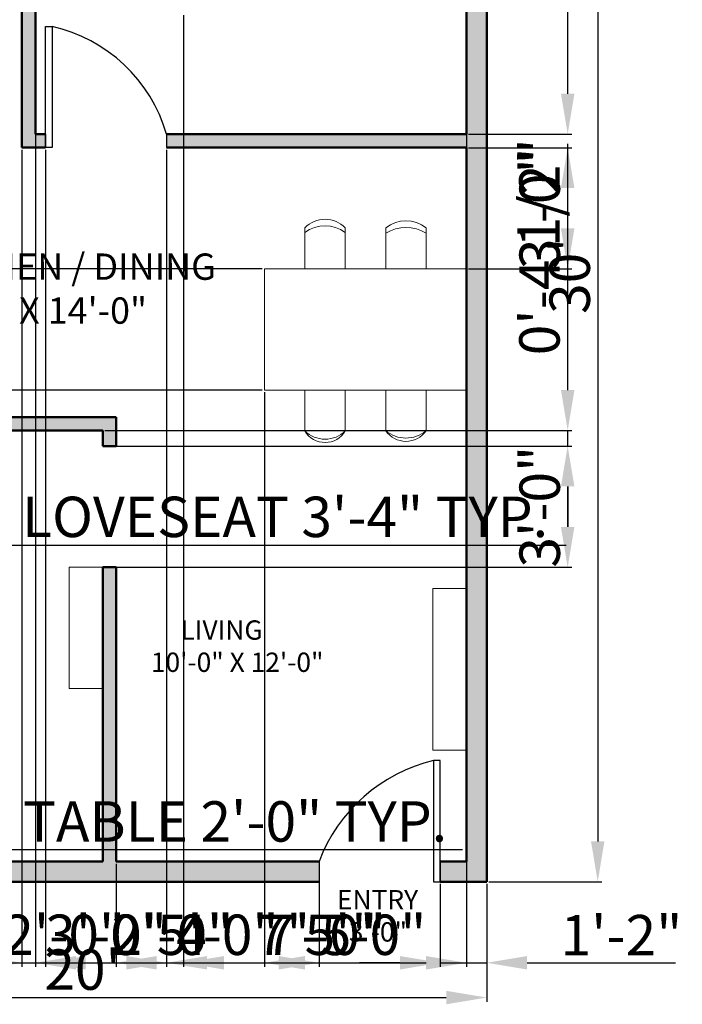
# Model space of a CAD drawing. Units: inches. Extents: x 2549 to 2991, y 1646 to 2183.
# Tile 2 of 3: x 2727 to 2924, y 1646 to 1938. Entities that reach past the tile are written whole.
import ezdxf

# ---------------------------------------------------------------- set-up
doc = ezdxf.new("R2010")
doc.units = ezdxf.units.IN
for name, color, linetype, lineweight in [('A-ANNO-DIMS', 2, 'Continuous', 18), ('A-ANNO-TEXT', 7, 'Continuous', 18), ('A-AREA-IDEN', 7, 'Continuous', 25), ('A-DOOR', 3, 'Continuous', 25), ('A-FURN', 9, 'Continuous', 18), ('A-WALL', 7, 'Continuous', 50)]:
    doc.layers.add(name, color=color, linetype=linetype, lineweight=lineweight)
doc.layers.add('A-WALL-PATT', color=251, linetype='Continuous', lineweight=13, true_color=0x636466)
doc.styles.get("Standard").update_dxf_attribs({"font": 'arial.ttf'})
doc.dimstyles.new('ISO-25', dxfattribs={"dimtxt": 12, "dimasz": 12, "dimexe": 1.25, "dimexo": 0.625, "dimtad": 1, "dimlunit": 3, "dimtxsty": 'Standard', "dimcen": 2.5, "dimadec": 0, "dimazin": 0, "dimtfac": 1, "dimtmove": 0, "dimatfit": 3, "dimfxl": 1, "dimarcsym": 0})

# ---------------------------------------------------------------- blocks, each defined once
blk = doc.blocks.new('*D5')
at = {"layer": 'A-ANNO-DIMS', "color": 0, "lineweight": -2, "transparency": 16777216}
for p, q in [((2866.66, 2042.26), (2900.26, 2042.26)), ((2899.01, 2030.26), (2899.01, 1694.26)), ((2866.66, 1682.26), (2900.26, 1682.26))]:
    blk.add_line(p, q, dxfattribs=at)
at = {"layer": 'A-ANNO-DIMS', "color": 0, "transparency": 16777216}
for points in [[(2897.01, 2030.26), (2901.01, 2030.26), (2899.01, 2042.26)], [(2897.01, 1694.26), (2901.01, 1694.26), (2899.01, 1682.26)]]:
    blk.add_solid(points, dxfattribs=at)
at = {"layer": 'Defpoints', "color": 0, "transparency": 16777216}
for p in [(2866.04, 2042.26), (2866.04, 1682.26), (2899.01, 1682.26)]:
    blk.add_point(p, dxfattribs=at)
at = {"layer": 'A-ANNO-DIMS', "color": 0, "transparency": 16777216, "insert": (2892.25, 1862.26), "char_height": 12, "attachment_point": 5, "rotation": 90}
blk.add_mtext("30'", dxfattribs=at)
blk = doc.blocks.new('*D13')
at = {"layer": 'A-ANNO-DIMS', "color": 0, "lineweight": -2, "transparency": 16777216}
for p, q in [((2626.04, 1681.64), (2626.04, 1646.63)), ((2866.04, 1681.64), (2866.04, 1646.63)), ((2638.04, 1647.88), (2854.04, 1647.88))]:
    blk.add_line(p, q, dxfattribs=at)
at = {"layer": 'A-ANNO-DIMS', "color": 0, "transparency": 16777216}
for points in [[(2638.04, 1649.88), (2638.04, 1645.88), (2626.04, 1647.88)], [(2854.04, 1649.88), (2854.04, 1645.88), (2866.04, 1647.88)]]:
    blk.add_solid(points, dxfattribs=at)
at = {"layer": 'Defpoints', "color": 0, "transparency": 16777216}
for p in [(2626.04, 1682.26), (2866.04, 1682.26), (2866.04, 1647.88)]:
    blk.add_point(p, dxfattribs=at)
at = {"layer": 'A-ANNO-DIMS', "color": 0, "transparency": 16777216, "insert": (2746.04, 1654.63), "char_height": 12, "attachment_point": 5}
blk.add_mtext("20'", dxfattribs=at)
blk = doc.blocks.new('*D16')
at = {"layer": 'A-ANNO-DIMS', "color": 0, "lineweight": -2, "transparency": 16777216}
for p, q in [((2670.52, 1787.63), (2670.52, 1780.98)), ((2710.65, 1787.63), (2710.65, 1780.98)), ((2682.52, 1782.23), (2698.65, 1782.23)), ((2710.65, 1782.23), (2889.68, 1782.23))]:
    blk.add_line(p, q, dxfattribs=at)
at = {"layer": 'A-ANNO-DIMS', "color": 0, "transparency": 16777216}
for points in [[(2682.52, 1784.23), (2682.52, 1780.23), (2670.52, 1782.23)], [(2698.65, 1784.23), (2698.65, 1780.23), (2710.65, 1782.23)]]:
    blk.add_solid(points, dxfattribs=at)
at = {"layer": 'Defpoints', "color": 0, "transparency": 16777216}
for p in [(2670.52, 1788.25), (2710.65, 1788.25), (2710.65, 1782.23)]:
    blk.add_point(p, dxfattribs=at)
at = {"layer": 'A-ANNO-DIMS', "color": 0, "transparency": 16777216, "insert": (2806.17, 1789.07), "char_height": 12, "attachment_point": 5}
blk.add_mtext('LOVESEAT 3\'-4" TYP.', dxfattribs=at)
blk = doc.blocks.new('*D17')
at = {"layer": 'A-ANNO-DIMS', "color": 0, "lineweight": -2, "transparency": 16777216}
for p, q in [((2716.67, 1820.92), (2716.67, 1934.15)), ((2711.28, 1808.92), (2717.92, 1808.92)), ((2716.67, 1788.25), (2716.67, 1808.92)), ((2711.28, 1788.25), (2717.92, 1788.25)), ((2716.67, 1776.25), (2716.67, 1764.25))]:
    blk.add_line(p, q, dxfattribs=at)
at = {"layer": 'A-ANNO-DIMS', "color": 0, "transparency": 16777216}
for points in [[(2714.67, 1820.92), (2718.67, 1820.92), (2716.67, 1808.92)], [(2714.67, 1776.25), (2718.67, 1776.25), (2716.67, 1788.25)]]:
    blk.add_solid(points, dxfattribs=at)
at = {"layer": 'Defpoints', "color": 0, "transparency": 16777216}
for p in [(2710.65, 1808.92), (2716.67, 1808.92), (2710.65, 1788.25)]:
    blk.add_point(p, dxfattribs=at)
at = {"layer": 'A-ANNO-DIMS', "color": 0, "transparency": 16777216, "insert": (2709.84, 1883.53), "char_height": 12, "attachment_point": 5, "rotation": 90}
blk.add_mtext('1\'-8 1/2" TYP.', dxfattribs=at)
blk = doc.blocks.new('*D18')
at = {"layer": 'A-ANNO-DIMS', "color": 0, "lineweight": -2, "transparency": 16777216}
for p, q in [((2639.3, 1694.84), (2639.3, 1690.62)), ((2663.3, 1694.84), (2663.3, 1690.62)), ((2627.3, 1691.87), (2615.3, 1691.87)), ((2639.3, 1691.87), (2663.3, 1691.87)), ((2675.3, 1691.87), (2858.88, 1691.87))]:
    blk.add_line(p, q, dxfattribs=at)
at = {"layer": 'A-ANNO-DIMS', "color": 0, "transparency": 16777216}
for points in [[(2627.3, 1693.87), (2627.3, 1689.87), (2639.3, 1691.87)], [(2675.3, 1693.87), (2675.3, 1689.87), (2663.3, 1691.87)]]:
    blk.add_solid(points, dxfattribs=at)
at = {"layer": 'Defpoints', "color": 0, "transparency": 16777216}
for p in [(2639.3, 1695.47), (2663.3, 1695.47), (2663.3, 1691.87)]:
    blk.add_point(p, dxfattribs=at)
at = {"layer": 'A-ANNO-DIMS', "color": 0, "transparency": 16777216, "insert": (2773.09, 1698.62), "char_height": 12, "attachment_point": 5}
blk.add_mtext('END TABLE 2\'-0" TYP.', dxfattribs=at)
blk = doc.blocks.new('*D30')
at = {"layer": 'A-ANNO-DIMS', "color": 0, "lineweight": -2, "transparency": 16777216}
for p, q in [((2852.26, 1681.64), (2852.26, 1656.96)), ((2866.04, 1681.64), (2866.04, 1656.96)), ((2840.26, 1658.21), (2828.26, 1658.21)), ((2852.26, 1658.21), (2866.04, 1658.21)), ((2878.04, 1658.21), (2922.06, 1658.21))]:
    blk.add_line(p, q, dxfattribs=at)
at = {"layer": 'A-ANNO-DIMS', "color": 0, "transparency": 16777216}
for points in [[(2840.26, 1660.21), (2840.26, 1656.21), (2852.26, 1658.21)], [(2878.04, 1660.21), (2878.04, 1656.21), (2866.04, 1658.21)]]:
    blk.add_solid(points, dxfattribs=at)
at = {"layer": 'Defpoints', "color": 0, "transparency": 16777216}
for p in [(2852.26, 1682.26), (2866.04, 1682.26), (2866.04, 1658.21)]:
    blk.add_point(p, dxfattribs=at)
at = {"layer": 'A-ANNO-DIMS', "color": 0, "transparency": 16777216, "insert": (2906.05, 1664.86), "char_height": 12, "attachment_point": 5}
blk.add_mtext('1\'-2"', dxfattribs=at)
blk = doc.blocks.new('*D33')
at = {"layer": 'A-ANNO-DIMS', "color": 0, "lineweight": -2, "transparency": 16777216}
for p, q in [((2675.89, 1963.64), (2675.89, 1656.96)), ((2699.89, 1963.64), (2699.89, 1656.96)), ((2663.89, 1658.21), (2651.89, 1658.21)), ((2675.89, 1658.21), (2699.89, 1658.21)), ((2711.89, 1658.21), (2757.24, 1658.21))]:
    blk.add_line(p, q, dxfattribs=at)
at = {"layer": 'A-ANNO-DIMS', "color": 0, "transparency": 16777216}
for points in [[(2663.89, 1660.21), (2663.89, 1656.21), (2675.89, 1658.21)], [(2711.89, 1660.21), (2711.89, 1656.21), (2699.89, 1658.21)]]:
    blk.add_solid(points, dxfattribs=at)
at = {"layer": 'Defpoints', "color": 0, "transparency": 16777216}
for p in [(2675.89, 1964.26), (2699.89, 1964.26), (2699.89, 1658.21)]:
    blk.add_point(p, dxfattribs=at)
at = {"layer": 'A-ANNO-DIMS', "color": 0, "transparency": 16777216, "insert": (2740.57, 1664.97), "char_height": 12, "attachment_point": 5}
blk.add_mtext('2\'-0"', dxfattribs=at)
blk = doc.blocks.new('*D35')
at = {"layer": 'A-ANNO-DIMS', "color": 0, "lineweight": -2, "transparency": 16777216}
for p, q in [((2734.98, 1899.64), (2734.98, 1656.96)), ((2770.98, 1899.64), (2770.98, 1656.96)), ((2746.98, 1658.21), (2758.98, 1658.21))]:
    blk.add_line(p, q, dxfattribs=at)
at = {"layer": 'A-ANNO-DIMS', "color": 0, "transparency": 16777216}
for points in [[(2746.98, 1660.21), (2746.98, 1656.21), (2734.98, 1658.21)], [(2758.98, 1660.21), (2758.98, 1656.21), (2770.98, 1658.21)]]:
    blk.add_solid(points, dxfattribs=at)
at = {"layer": 'Defpoints', "color": 0, "transparency": 16777216}
for p in [(2734.98, 1900.26), (2770.98, 1900.26), (2770.98, 1658.21)]:
    blk.add_point(p, dxfattribs=at)
at = {"layer": 'A-ANNO-DIMS', "color": 0, "transparency": 16777216, "insert": (2752.98, 1664.97), "char_height": 12, "attachment_point": 5}
blk.add_mtext('3\'-0"', dxfattribs=at)
blk = doc.blocks.new('*D36')
at = {"layer": 'A-ANNO-DIMS', "color": 0, "lineweight": -2, "transparency": 16777216}
for p, q in [((2752.66, 1811.65), (2891.34, 1811.65)), ((2890.09, 1787.65), (2890.09, 1799.65)), ((2752.66, 1775.65), (2891.34, 1775.65))]:
    blk.add_line(p, q, dxfattribs=at)
at = {"layer": 'A-ANNO-DIMS', "color": 0, "transparency": 16777216}
for points in [[(2888.09, 1799.65), (2892.09, 1799.65), (2890.09, 1811.65)], [(2888.09, 1787.65), (2892.09, 1787.65), (2890.09, 1775.65)]]:
    blk.add_solid(points, dxfattribs=at)
at = {"layer": 'Defpoints', "color": 0, "transparency": 16777216}
for p in [(2752.04, 1811.65), (2890.09, 1811.65), (2752.04, 1775.65)]:
    blk.add_point(p, dxfattribs=at)
at = {"layer": 'A-ANNO-DIMS', "color": 0, "transparency": 16777216, "insert": (2883.33, 1793.65), "char_height": 12, "attachment_point": 5, "rotation": 90}
blk.add_mtext('3\'-0"', dxfattribs=at)
blk = doc.blocks.new('*D37')
at = {"layer": 'A-ANNO-DIMS', "color": 0, "lineweight": -2, "transparency": 16777216}
for p, q in [((2770.98, 1899.64), (2770.98, 1656.96)), ((2860.04, 1899.64), (2860.04, 1656.96)), ((2782.98, 1658.21), (2848.04, 1658.21))]:
    blk.add_line(p, q, dxfattribs=at)
at = {"layer": 'A-ANNO-DIMS', "color": 0, "transparency": 16777216}
for points in [[(2782.98, 1660.21), (2782.98, 1656.21), (2770.98, 1658.21)], [(2848.04, 1660.21), (2848.04, 1656.21), (2860.04, 1658.21)]]:
    blk.add_solid(points, dxfattribs=at)
at = {"layer": 'Defpoints', "color": 0, "transparency": 16777216}
for p in [(2770.98, 1900.26), (2860.04, 1900.26), (2860.04, 1658.21)]:
    blk.add_point(p, dxfattribs=at)
at = {"layer": 'A-ANNO-DIMS', "color": 0, "transparency": 16777216, "insert": (2815.51, 1664.94), "char_height": 12, "attachment_point": 5}
blk.add_mtext('7\'-5"', dxfattribs=at)
blk = doc.blocks.new('*D38')
at = {"layer": 'A-ANNO-DIMS', "color": 0, "lineweight": -2, "transparency": 16777216}
for p, q in [((2890.09, 1828.26), (2890.09, 1901.37)), ((2752.66, 1816.26), (2891.34, 1816.26)), ((2890.09, 1811.65), (2890.09, 1816.26)), ((2752.66, 1811.65), (2891.34, 1811.65)), ((2890.09, 1799.65), (2890.09, 1787.65))]:
    blk.add_line(p, q, dxfattribs=at)
at = {"layer": 'A-ANNO-DIMS', "color": 0, "transparency": 16777216}
for points in [[(2888.09, 1828.26), (2892.09, 1828.26), (2890.09, 1816.26)], [(2888.09, 1799.65), (2892.09, 1799.65), (2890.09, 1811.65)]]:
    blk.add_solid(points, dxfattribs=at)
at = {"layer": 'Defpoints', "color": 0, "transparency": 16777216}
for p in [(2752.04, 1816.26), (2890.09, 1816.26), (2752.04, 1811.65)]:
    blk.add_point(p, dxfattribs=at)
at = {"layer": 'A-ANNO-DIMS', "color": 0, "transparency": 16777216, "insert": (2883.26, 1870.82), "char_height": 12, "attachment_point": 5, "rotation": 90}
blk.add_mtext('0\'-4 1/2"', dxfattribs=at)
blk = doc.blocks.new('*D39')
at = {"layer": 'A-ANNO-DIMS', "color": 0, "lineweight": -2, "transparency": 16777216}
for p, q in [((2800.04, 1827.64), (2800.04, 1656.96)), ((2860.04, 1827.64), (2860.04, 1656.96)), ((2812.04, 1658.21), (2848.04, 1658.21))]:
    blk.add_line(p, q, dxfattribs=at)
at = {"layer": 'A-ANNO-DIMS', "color": 0, "transparency": 16777216}
for points in [[(2812.04, 1660.21), (2812.04, 1656.21), (2800.04, 1658.21)], [(2848.04, 1660.21), (2848.04, 1656.21), (2860.04, 1658.21)]]:
    blk.add_solid(points, dxfattribs=at)
at = {"layer": 'Defpoints', "color": 0, "transparency": 16777216}
for p in [(2800.04, 1828.26), (2860.04, 1828.26), (2860.04, 1658.21)]:
    blk.add_point(p, dxfattribs=at)
at = {"layer": 'A-ANNO-DIMS', "color": 0, "transparency": 16777216, "insert": (2830.04, 1664.97), "char_height": 12, "attachment_point": 5}
blk.add_mtext('5\'-0"', dxfattribs=at)
blk = doc.blocks.new('*D40')
at = {"layer": 'A-ANNO-DIMS', "color": 0, "lineweight": -2, "transparency": 16777216}
for p, q in [((2799.41, 1864.26), (2600.74, 1864.26)), ((2601.99, 1840.26), (2601.99, 1852.26)), ((2799.41, 1828.26), (2600.74, 1828.26))]:
    blk.add_line(p, q, dxfattribs=at)
at = {"layer": 'A-ANNO-DIMS', "color": 0, "transparency": 16777216}
for points in [[(2599.99, 1852.26), (2603.99, 1852.26), (2601.99, 1864.26)], [(2599.99, 1840.26), (2603.99, 1840.26), (2601.99, 1828.26)]]:
    blk.add_solid(points, dxfattribs=at)
at = {"layer": 'Defpoints', "color": 0, "transparency": 16777216}
for p in [(2601.99, 1864.26), (2800.04, 1864.26), (2800.04, 1828.26)]:
    blk.add_point(p, dxfattribs=at)
at = {"layer": 'A-ANNO-DIMS', "color": 0, "transparency": 16777216, "insert": (2595.23, 1846.26), "char_height": 12, "attachment_point": 5, "rotation": 90}
blk.add_mtext('3\'-0"', dxfattribs=at)
blk = doc.blocks.new('*D42')
at = {"layer": 'A-ANNO-DIMS', "color": 0, "lineweight": -2, "transparency": 16777216}
for p, q in [((2776.04, 1939.64), (2776.04, 1656.96)), ((2860.04, 1939.64), (2860.04, 1656.96)), ((2788.04, 1658.21), (2848.04, 1658.21))]:
    blk.add_line(p, q, dxfattribs=at)
at = {"layer": 'A-ANNO-DIMS', "color": 0, "transparency": 16777216}
for points in [[(2788.04, 1660.21), (2788.04, 1656.21), (2776.04, 1658.21)], [(2848.04, 1660.21), (2848.04, 1656.21), (2860.04, 1658.21)]]:
    blk.add_solid(points, dxfattribs=at)
at = {"layer": 'Defpoints', "color": 0, "transparency": 16777216}
for p in [(2776.04, 1940.26), (2860.04, 1940.26), (2860.04, 1658.21)]:
    blk.add_point(p, dxfattribs=at)
at = {"layer": 'A-ANNO-DIMS', "color": 0, "transparency": 16777216, "insert": (2818.04, 1664.97), "char_height": 12, "attachment_point": 5}
blk.add_mtext('7\'-0"', dxfattribs=at)
blk = doc.blocks.new('*D44')
at = {"layer": 'A-ANNO-DIMS', "color": 0, "lineweight": -2, "transparency": 16777216}
for p, q in [((2708.04, 1963.64), (2708.04, 1656.96)), ((2732.04, 1963.64), (2732.04, 1656.96)), ((2696.04, 1658.21), (2684.04, 1658.21)), ((2708.04, 1658.21), (2732.04, 1658.21)), ((2744.04, 1658.21), (2789.39, 1658.21))]:
    blk.add_line(p, q, dxfattribs=at)
at = {"layer": 'A-ANNO-DIMS', "color": 0, "transparency": 16777216}
for points in [[(2696.04, 1660.21), (2696.04, 1656.21), (2708.04, 1658.21)], [(2744.04, 1660.21), (2744.04, 1656.21), (2732.04, 1658.21)]]:
    blk.add_solid(points, dxfattribs=at)
at = {"layer": 'Defpoints', "color": 0, "transparency": 16777216}
for p in [(2708.04, 1964.26), (2732.04, 1964.26), (2732.04, 1658.21)]:
    blk.add_point(p, dxfattribs=at)
at = {"layer": 'A-ANNO-DIMS', "color": 0, "transparency": 16777216, "insert": (2772.72, 1664.97), "char_height": 12, "attachment_point": 5}
blk.add_mtext('2\'-0"', dxfattribs=at)
blk = doc.blocks.new('*D45')
at = {"layer": 'A-ANNO-DIMS', "color": 0, "lineweight": -2, "transparency": 16777216}
for p, q in [((2860.66, 2036.26), (2891.34, 2036.26)), ((2890.09, 1916.26), (2890.09, 2024.26)), ((2860.66, 1904.26), (2891.34, 1904.26))]:
    blk.add_line(p, q, dxfattribs=at)
at = {"layer": 'A-ANNO-DIMS', "color": 0, "transparency": 16777216}
for points in [[(2888.09, 2024.26), (2892.09, 2024.26), (2890.09, 2036.26)], [(2888.09, 1916.26), (2892.09, 1916.26), (2890.09, 1904.26)]]:
    blk.add_solid(points, dxfattribs=at)
at = {"layer": 'Defpoints', "color": 0, "transparency": 16777216}
for p in [(2860.04, 2036.26), (2890.09, 2036.26), (2860.04, 1904.26)]:
    blk.add_point(p, dxfattribs=at)
at = {"layer": 'A-ANNO-DIMS', "color": 0, "transparency": 16777216, "insert": (2883.34, 1970.26), "char_height": 12, "attachment_point": 5, "rotation": 90}
blk.add_mtext('11\'-0"', dxfattribs=at)
blk = doc.blocks.new('*D47')
at = {"layer": 'A-ANNO-DIMS', "color": 0, "lineweight": -2, "transparency": 16777216}
for p, q in [((2860.66, 1900.26), (2891.34, 1900.26)), ((2890.09, 1876.26), (2890.09, 1888.26)), ((2860.66, 1864.26), (2891.34, 1864.26))]:
    blk.add_line(p, q, dxfattribs=at)
at = {"layer": 'A-ANNO-DIMS', "color": 0, "transparency": 16777216}
for points in [[(2888.09, 1888.26), (2892.09, 1888.26), (2890.09, 1900.26)], [(2888.09, 1876.26), (2892.09, 1876.26), (2890.09, 1864.26)]]:
    blk.add_solid(points, dxfattribs=at)
at = {"layer": 'Defpoints', "color": 0, "transparency": 16777216}
for p in [(2860.04, 1900.26), (2890.09, 1900.26), (2860.04, 1864.26)]:
    blk.add_point(p, dxfattribs=at)
at = {"layer": 'A-ANNO-DIMS', "color": 0, "transparency": 16777216, "insert": (2883.33, 1882.26), "char_height": 12, "attachment_point": 5, "rotation": 90}
blk.add_mtext('3\'-0"', dxfattribs=at)
blk = doc.blocks.new('*D48')
at = {"layer": 'A-ANNO-DIMS', "color": 0, "lineweight": -2, "transparency": 16777216}
for p, q in [((2756.04, 1687.64), (2756.04, 1656.96)), ((2816.26, 1687.64), (2816.26, 1656.96)), ((2768.04, 1658.21), (2804.26, 1658.21))]:
    blk.add_line(p, q, dxfattribs=at)
at = {"layer": 'A-ANNO-DIMS', "color": 0, "transparency": 16777216}
for points in [[(2768.04, 1660.21), (2768.04, 1656.21), (2756.04, 1658.21)], [(2804.26, 1660.21), (2804.26, 1656.21), (2816.26, 1658.21)]]:
    blk.add_solid(points, dxfattribs=at)
at = {"layer": 'Defpoints', "color": 0, "transparency": 16777216}
for p in [(2756.04, 1688.26), (2816.26, 1688.26), (2816.26, 1658.21)]:
    blk.add_point(p, dxfattribs=at)
at = {"layer": 'A-ANNO-DIMS', "color": 0, "transparency": 16777216, "insert": (2786.15, 1664.97), "char_height": 12, "attachment_point": 5}
blk.add_mtext('5\'-0"', dxfattribs=at)
blk = doc.blocks.new('*D49')
at = {"layer": 'A-ANNO-DIMS', "color": 0, "lineweight": -2, "transparency": 16777216}
for p, q in [((2732.04, 1903.64), (2732.04, 1656.96)), ((2728.04, 1899.64), (2728.04, 1656.96)), ((2716.04, 1658.21), (2704.04, 1658.21)), ((2728.04, 1658.21), (2732.04, 1658.21)), ((2744.04, 1658.21), (2789.19, 1658.21))]:
    blk.add_line(p, q, dxfattribs=at)
at = {"layer": 'A-ANNO-DIMS', "color": 0, "transparency": 16777216}
for points in [[(2716.04, 1660.21), (2716.04, 1656.21), (2728.04, 1658.21)], [(2744.04, 1660.21), (2744.04, 1656.21), (2732.04, 1658.21)]]:
    blk.add_solid(points, dxfattribs=at)
at = {"layer": 'Defpoints', "color": 0, "transparency": 16777216}
for p in [(2732.04, 1904.26), (2728.04, 1900.26), (2732.04, 1658.21)]:
    blk.add_point(p, dxfattribs=at)
at = {"layer": 'A-ANNO-DIMS', "color": 0, "transparency": 16777216, "insert": (2772.61, 1664.97), "char_height": 12, "attachment_point": 5}
blk.add_mtext('0\'-4"', dxfattribs=at)

msp = doc.modelspace()

# ---------------------------------------------------------------- hatches: boundary and pattern name
at = {"layer": 'A-WALL-PATT'}
h = msp.add_hatch(color=256, dxfattribs=at)
h.dxf.hatch_style = 1
h.paths.add_polyline_path([(2765.46, 2042.264), (2626.038, 2042.264), (2626.038, 1682.264), (2673.991, 1682.264), (2673.991, 1688.264), (2632.038, 1688.264), (2632.038, 1816.264), (2752.038, 1816.264), (2752.038, 1811.649), (2756.038, 1811.649), (2756.038, 1820.264), (2632.038, 1820.264), (2632.038, 1960.264), (2675.89, 1960.264), (2675.89, 1964.264), (2632.038, 1964.264), (2632.038, 2036.264), (2704.038, 2036.264), (2704.038, 1964.264), (2699.89, 1964.264), (2699.89, 1960.264), (2728.038, 1960.264), (2728.038, 1900.264), (2734.981, 1900.264), (2734.981, 1904.264), (2732.038, 1904.264), (2732.038, 1964.264), (2708.038, 1964.264), (2708.038, 2036.264), (2765.46, 2036.264)])
h.paths.add_polyline_path([(2866.038, 2042.264), (2825.46, 2042.264), (2825.46, 2036.264), (2860.038, 2036.264), (2860.038, 1904.264), (2770.981, 1904.264), (2770.981, 1900.264), (2860.038, 1900.264), (2860.038, 1688.264), (2852.256, 1688.264), (2852.256, 1682.264), (2866.038, 1682.264)])
h.paths.add_polyline_path([(2816.256, 1688.264), (2756.038, 1688.264), (2756.038, 1775.649), (2752.038, 1775.649), (2752.038, 1688.264), (2721.991, 1688.264), (2721.991, 1682.264), (2816.256, 1682.264)])

# ---------------------------------------------------------------- linework, layer by layer
at = {"layer": 'A-DOOR'}
for p, q in [((2734.981, 1900.264), (2734.981, 1936.264)), ((2734.981, 1936.264), (2736.981, 1936.264)), ((2736.981, 1936.264), (2736.981, 1900.264)), ((2734.981, 1904.264), (2734.981, 1900.264)), ((2770.981, 1904.264), (2770.981, 1900.264)), ((2736.981, 1900.264), (2734.981, 1900.264)), ((2852.256, 1718.264), (2850.256, 1718.264)), ((2850.256, 1718.264), (2850.256, 1682.264)), ((2852.256, 1682.264), (2852.256, 1718.264)), ((2816.256, 1688.264), (2816.256, 1682.264)), ((2852.256, 1688.264), (2852.256, 1682.264)), ((2850.256, 1682.264), (2852.256, 1682.264))]:
    msp.add_line(p, q, dxfattribs=at)
for centre, radius, start, end in [((2726.788, 1891.372), 46.035, 16.26336, 77.20805), ((2861.526, 1671.224), 48.371, 103.47383, 159.3735)]:
    msp.add_arc(centre, radius, start, end, dxfattribs=at)
at = {"layer": 'A-FURN'}
for p, q in [((2812.055, 1876.434), (2812.055, 1864.264)), ((2824.055, 1876.434), (2824.055, 1864.264)), ((2836.055, 1876.434), (2836.055, 1864.264)), ((2848.055, 1876.434), (2848.055, 1864.264)), ((2800.038, 1864.264), (2860.038, 1864.264)), ((2800.038, 1864.264), (2800.038, 1828.264)), ((2800.038, 1828.264), (2860.038, 1828.264)), ((2812.055, 1828.358), (2812.055, 1816.188)), ((2824.055, 1828.358), (2824.055, 1816.188)), ((2836.055, 1828.358), (2836.055, 1816.188)), ((2848.055, 1828.358), (2848.055, 1816.188)), ((2752.038, 1775.649), (2742.038, 1775.649)), ((2742.038, 1775.649), (2742.038, 1739.649)), ((2860.038, 1769.373), (2850.038, 1769.373)), ((2850.038, 1769.373), (2850.038, 1721.373)), ((2742.038, 1739.649), (2752.038, 1739.649)), ((2860.038, 1721.373), (2850.038, 1721.373))]:
    msp.add_line(p, q, dxfattribs=at)
for centre, radius, start, end in [((2818.055, 1870.647), 8.336, 43.96332, 136.03668), ((2842.055, 1868.889), 9.64, 51.507, 128.493), ((2818.055, 1867.024), 10.018, 53.20577, 126.79423), ((2842.055, 1865.115), 11.451, 58.40203, 121.59797), ((2818.055, 1819.624), 6.914, 209.79606, 330.20394), ((2818.055, 1822.121), 8.438, 224.68008, 315.31992), ((2842.055, 1820.334), 7.293, 214.64452, 325.35548), ((2842.055, 1823.391), 9.375, 230.20798, 309.79202)]:
    msp.add_arc(centre, radius, start, end, dxfattribs=at)
at = {"layer": 'A-WALL'}
for p, q in [((2866.038, 2042.264), (2866.038, 1682.264)), ((2860.038, 2036.264), (2860.038, 1904.264)), ((2732.038, 1964.264), (2732.038, 1904.264)), ((2728.038, 1960.264), (2728.038, 1900.264)), ((2732.038, 1904.264), (2734.981, 1904.264)), ((2770.981, 1904.264), (2860.038, 1904.264)), ((2728.038, 1900.264), (2734.981, 1900.264)), ((2770.981, 1900.264), (2860.038, 1900.264)), ((2860.038, 1900.264), (2860.038, 1688.264)), ((2632.038, 1820.264), (2756.038, 1820.264)), ((2756.038, 1811.649), (2756.038, 1820.264)), ((2632.038, 1816.264), (2752.038, 1816.264)), ((2752.038, 1811.649), (2752.038, 1816.264)), ((2752.038, 1811.649), (2756.038, 1811.649)), ((2752.038, 1688.264), (2752.038, 1775.649)), ((2752.038, 1775.649), (2756.038, 1775.649)), ((2756.038, 1688.264), (2756.038, 1775.649)), ((2752.038, 1688.264), (2632.038, 1688.264)), ((2816.256, 1688.264), (2756.038, 1688.264)), ((2860.038, 1688.264), (2852.256, 1688.264)), ((2816.256, 1682.264), (2626.038, 1682.264)), ((2866.038, 1682.264), (2852.256, 1682.264))]:
    msp.add_line(p, q, dxfattribs=at)

# ---------------------------------------------------------------- texts
at = {"layer": 'A-ANNO-TEXT', "insert": (2819.835, 1679.815), "char_height": 5.7375, "attachment_point": 1}
msp.add_mtext_dynamic_manual_height_columns(' ENTRY \\P   3\'-0"', width=199.71745, gutter_width=28.687, heights=[0], dxfattribs=at)
at = {"layer": 'A-AREA-IDEN', "attachment_point": 1}
for s, width, gutter_width, insert, char_height in [('KITCHEN / DINING\\P12\'-0" X 14\'-0"', 272.27661, 39.11, (2695.29, 1868.84), 7.82199), ('     LIVING\\P10\'-0" X 12\'-0"', 199.71745, 28.687, (2766.318, 1759.89), 5.7375)]:
    msp.add_mtext_dynamic_manual_height_columns(s, width=width, gutter_width=gutter_width, heights=[0], dxfattribs=dict(at, insert=insert, char_height=char_height))

# ---------------------------------------------------------------- dimensions: what is measured, and where the dimension line sits
at = {"layer": 'A-ANNO-DIMS'}
for base, p1, p2, override, picture, middle in [((2899.007, 1682.264), (2866.038, 2042.264), (2866.038, 1682.264), {"dimclrd": 0, "dimclre": 0, "dimclrt": 0}, '*D5', (2892.251, 1862.264)), ((2890.088, 2036.264), (2860.038, 1904.264), (2860.038, 2036.264), {"dimdec": 1, "dimlfac": 1, "dimrnd": 0, "dimzin": 1, "dimdsep": 46, "dimlunit": 4, "dimfrac": 2}, '*D45', (2883.336, 1970.264)), ((2890.088, 1816.264), (2752.038, 1811.649), (2752.038, 1816.264), {"dimdec": 1, "dimlfac": 1, "dimrnd": 0, "dimzin": 1, "dimdsep": 46, "dimlunit": 4, "dimfrac": 2}, '*D38', (2883.259, 1870.819)), ((2890.088, 1900.264), (2860.038, 1864.264), (2860.038, 1900.264), {"dimdec": 1, "dimlfac": 1, "dimrnd": 0, "dimzin": 1, "dimdsep": 46, "dimlunit": 4, "dimfrac": 2}, '*D47', (2883.332, 1882.264)), ((2601.988, 1864.264), (2800.038, 1828.264), (2800.038, 1864.264), {"dimdec": 1, "dimlfac": 1, "dimrnd": 0, "dimzin": 1, "dimdsep": 46, "dimlunit": 4, "dimfrac": 2}, '*D40', (2595.232, 1846.264)), ((2890.088, 1811.649), (2752.038, 1775.649), (2752.038, 1811.649), {"dimdec": 1, "dimlfac": 1, "dimrnd": 0, "dimzin": 1, "dimdsep": 46, "dimlunit": 4, "dimfrac": 2}, '*D36', (2883.332, 1793.649))]:
    dim = msp.add_linear_dim(base=base, p1=p1, p2=p2, angle=90, dimstyle='ISO-25', override=override, dxfattribs=at)
    dim.commit()
    dim.dimension.update_dxf_attribs({"geometry": picture, "text_midpoint": middle})
for base, p1, p2, override, picture, middle in [((2699.89, 1658.214), (2675.89, 1964.264), (2699.89, 1964.264), {"dimdec": 1, "dimlfac": 1, "dimrnd": 0, "dimzin": 1, "dimdsep": 46, "dimlunit": 4, "dimfrac": 2}, '*D33', (2740.567, 1664.966)), ((2732.038, 1658.214), (2708.038, 1964.264), (2732.038, 1964.264), {"dimdec": 1, "dimlfac": 1, "dimrnd": 0, "dimzin": 1, "dimdsep": 46, "dimlunit": 4, "dimfrac": 2}, '*D44', (2772.715, 1664.966)), ((2860.038, 1658.214), (2776.038, 1940.264), (2860.038, 1940.264), {"dimdec": 1, "dimlfac": 1, "dimrnd": 0, "dimzin": 1, "dimdsep": 46, "dimlunit": 4, "dimfrac": 2}, '*D42', (2818.038, 1664.966)), ((2732.038, 1658.214), (2728.038, 1900.264), (2732.038, 1904.264), {"dimdec": 1, "dimlfac": 1, "dimrnd": 0, "dimzin": 1, "dimdsep": 46, "dimlunit": 4, "dimfrac": 2}, '*D49', (2772.613, 1664.966)), ((2770.981, 1658.214), (2734.981, 1900.264), (2770.981, 1900.264), {"dimdec": 1, "dimlfac": 1, "dimrnd": 0, "dimzin": 1, "dimdsep": 46, "dimlunit": 4, "dimfrac": 2}, '*D35', (2752.981, 1664.97)), ((2860.038, 1658.214), (2770.981, 1900.264), (2860.038, 1900.264), {"dimdec": 1, "dimlfac": 1, "dimrnd": 0, "dimzin": 1, "dimdsep": 46, "dimlunit": 4, "dimfrac": 2}, '*D37', (2815.51, 1664.941)), ((2860.038, 1658.214), (2800.038, 1828.264), (2860.038, 1828.264), {"dimdec": 1, "dimlfac": 1, "dimrnd": 0, "dimzin": 1, "dimdsep": 46, "dimlunit": 4, "dimfrac": 2}, '*D39', (2830.038, 1664.966)), ((2816.256, 1658.214), (2756.038, 1688.264), (2816.256, 1688.264), {"dimdec": 1, "dimlfac": 1, "dimrnd": 0, "dimzin": 1, "dimdsep": 46, "dimlunit": 4, "dimfrac": 2}, '*D48', (2786.147, 1664.966)), ((2866.038, 1647.88), (2626.038, 1682.264), (2866.038, 1682.264), {"dimclrd": 0, "dimclre": 0, "dimclrt": 0}, '*D13', (2746.038, 1654.632)), ((2866.038, 1658.214), (2852.256, 1682.264), (2866.038, 1682.264), {"dimdec": 1, "dimlfac": 1, "dimrnd": 0, "dimzin": 1, "dimdsep": 46, "dimlunit": 4, "dimfrac": 2}, '*D30', (2906.048, 1664.864))]:
    dim = msp.add_linear_dim(base=base, p1=p1, p2=p2, dimstyle='ISO-25', override=override, dxfattribs=at)
    dim.commit()
    dim.dimension.update_dxf_attribs({"geometry": picture, "text_midpoint": middle})
dim = msp.add_linear_dim(base=(2716.671, 1808.918), p1=(2710.651, 1788.253), p2=(2710.651, 1808.918), angle=90, text='<> TYP.', dimstyle='ISO-25', override={"dimdec": 1, "dimlfac": 1, "dimrnd": 0, "dimzin": 1, "dimdsep": 46, "dimlunit": 4, "dimfrac": 2}, dxfattribs=at)
dim.commit()
dim.dimension.update_dxf_attribs({"geometry": '*D17', "text_midpoint": (2709.841, 1883.532)})
for base, p1, p2, text, picture, middle in [((2710.651, 1782.233), (2670.518, 1788.253), (2710.651, 1788.253), 'LOVESEAT <> TYP.', '*D16', (2806.167, 1789.071)), ((2663.3, 1691.869), (2639.3, 1695.469), (2663.3, 1695.469), 'END TABLE <> TYP.', '*D18', (2773.092, 1698.62))]:
    dim = msp.add_linear_dim(base=base, p1=p1, p2=p2, text=text, dimstyle='ISO-25', override={"dimdec": 1, "dimlfac": 1, "dimrnd": 0, "dimzin": 1, "dimdsep": 46, "dimlunit": 4, "dimfrac": 2}, dxfattribs=at)
    dim.commit()
    dim.dimension.update_dxf_attribs({"geometry": picture, "text_midpoint": middle})

doc.saveas('drawing.dxf')
